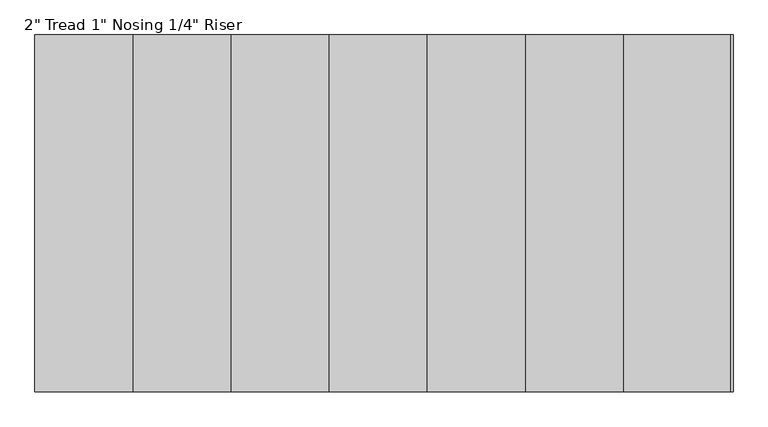
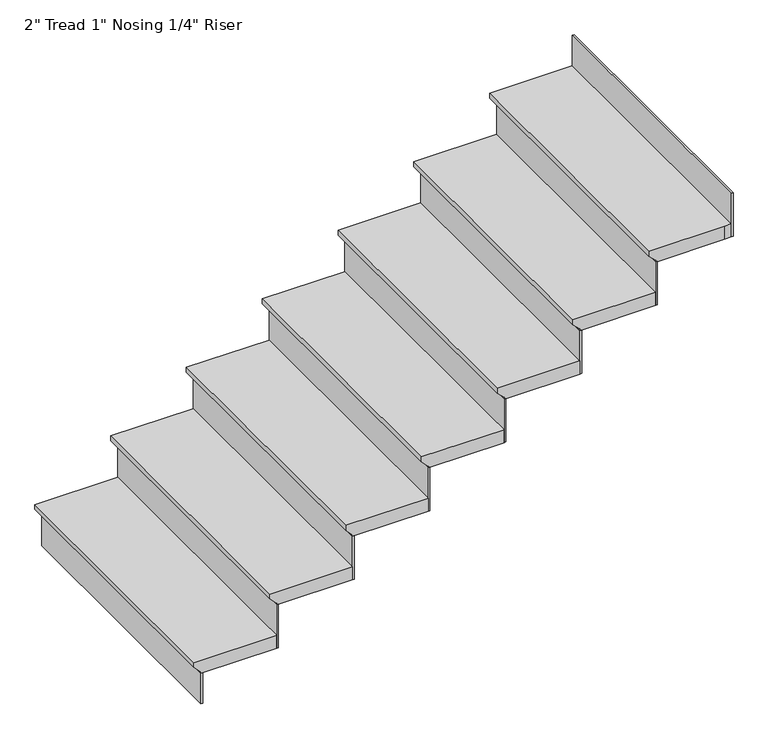
"""IFC4 building model written with IfcOpenShell, lengths in millimetres: stair flight geometry."""

from ifc_helpers import new_model, si_unit, origin, place, context, project, spatial, faceted_brep, source, transform, mapped, element, save


def stair_flight_c1e9d316(model_context):
    return source(origin(), model_context, "Body", "Brep", [
        faceted_brep([(-8426.5655018, -682.6966995, 150.2833333), (-8426.5655018, -682.6966995, 169.3333333), (-8426.5655018, 332.8576368, 169.3333333), (-8426.5655018, 332.8576368, 150.2833333), (-8401.1655018, -682.6966995, 124.8833333), (-8401.1655018, 332.8576368, 124.8833333), (-8121.7655018, -682.6966995, 169.3333333), (-8121.7655018, 332.8576368, 169.3333333), (-8401.1655018, 332.8576368, 118.5333333), (-8121.7655018, 332.8576368, 118.5333333), (-8121.7655018, -682.6966995, 118.5333333), (-8401.1655018, -682.6966995, 118.5333333)], [[[0, 1, 2, 3]], [[4, 0, 3, 5]], [[2, 1, 6, 7]], [[8, 9, 10, 11]], [[2, 7, 9, 8, 5, 3]], [[8, 11, 4, 5]], [[6, 1, 0, 4, 11, 10]], [[7, 6, 10, 9]]]),
        faceted_brep([(-8401.1655018, -682.6966995, 118.5333333), (-8401.1655018, -682.6966995, 0.0), (-8394.8155018, -682.6966995, 0.0), (-8394.8155018, -682.6966995, 118.5333333), (-8401.1655018, 332.8576368, 118.5333333), (-8394.8155018, 332.8576368, 118.5333333), (-8394.8155018, 332.8576368, 0.0), (-8401.1655018, 332.8576368, 0.0)], [[[0, 1, 2, 3]], [[4, 5, 6, 7]], [[1, 0, 4, 7]], [[2, 1, 7, 6]], [[3, 2, 6, 5]], [[0, 3, 5, 4]]]),
        faceted_brep([(-6445.3655018, -682.6966995, 1303.8666667), (-6445.3655018, -682.6966995, 1134.5333333), (-6439.0155018, -682.6966995, 1134.5333333), (-6439.0155018, -682.6966995, 1303.8666667), (-6445.3655018, 332.8576368, 1303.8666667), (-6439.0155018, 332.8576368, 1303.8666667), (-6439.0155018, 332.8576368, 1134.5333333), (-6445.3655018, 332.8576368, 1134.5333333)], [[[0, 1, 2, 3]], [[4, 5, 6, 7]], [[1, 0, 4, 7]], [[2, 1, 7, 6]], [[3, 2, 6, 5]], [[0, 3, 5, 4]]]),
        faceted_brep([(-8121.7655018, -682.6966995, 287.8666667), (-8121.7655018, -682.6966995, 118.5333333), (-8115.4155018, -682.6966995, 118.5333333), (-8115.4155018, -682.6966995, 287.8666667), (-8121.7655018, 332.8576368, 287.8666667), (-8115.4155018, 332.8576368, 287.8666667), (-8115.4155018, 332.8576368, 118.5333333), (-8121.7655018, 332.8576368, 118.5333333)], [[[0, 1, 2, 3]], [[4, 5, 6, 7]], [[1, 0, 4, 7]], [[2, 1, 7, 6]], [[3, 2, 6, 5]], [[0, 3, 5, 4]]]),
        faceted_brep([(-8147.1655018, 332.8576368, 338.6666667), (-8147.1655018, -682.6966995, 338.6666667), (-7842.3655018, -682.6966995, 338.6666667), (-7842.3655018, 332.8576368, 338.6666667), (-8121.7655018, 332.8576368, 287.8666667), (-7842.3655018, 332.8576368, 287.8666667), (-7842.3655018, -682.6966995, 287.8666667), (-8121.7655018, -682.6966995, 287.8666667), (-8121.7655018, 332.8576368, 294.2166667), (-8147.1655018, 332.8576368, 319.6166667), (-8121.7655018, -682.6966995, 294.2166667), (-8147.1655018, -682.6966995, 319.6166667)], [[[0, 1, 2, 3]], [[4, 5, 6, 7]], [[0, 3, 5, 4, 8, 9]], [[4, 7, 10, 8]], [[2, 1, 11, 10, 7, 6]], [[3, 2, 6, 5]], [[11, 1, 0, 9]], [[10, 11, 9, 8]]]),
        faceted_brep([(-7842.3655018, -682.6966995, 457.2), (-7842.3655018, -682.6966995, 287.8666667), (-7836.0155018, -682.6966995, 287.8666667), (-7836.0155018, -682.6966995, 457.2), (-7842.3655018, 332.8576368, 457.2), (-7836.0155018, 332.8576368, 457.2), (-7836.0155018, 332.8576368, 287.8666667), (-7842.3655018, 332.8576368, 287.8666667)], [[[0, 1, 2, 3]], [[4, 5, 6, 7]], [[1, 0, 4, 7]], [[2, 1, 7, 6]], [[3, 2, 6, 5]], [[0, 3, 5, 4]]]),
        faceted_brep([(-7867.7655018, 332.8576368, 508.0), (-7867.7655018, -682.6966995, 508.0), (-7562.9655018, -682.6966995, 508.0), (-7562.9655018, 332.8576368, 508.0), (-7842.3655018, 332.8576368, 457.2), (-7562.9655018, 332.8576368, 457.2), (-7562.9655018, -682.6966995, 457.2), (-7842.3655018, -682.6966995, 457.2), (-7842.3655018, 332.8576368, 463.55), (-7867.7655018, 332.8576368, 488.95), (-7842.3655018, -682.6966995, 463.55), (-7867.7655018, -682.6966995, 488.95)], [[[0, 1, 2, 3]], [[4, 5, 6, 7]], [[0, 3, 5, 4, 8, 9]], [[4, 7, 10, 8]], [[2, 1, 11, 10, 7, 6]], [[3, 2, 6, 5]], [[11, 1, 0, 9]], [[10, 11, 9, 8]]]),
        faceted_brep([(-7562.9655018, -682.6966995, 626.5333333), (-7562.9655018, -682.6966995, 457.2), (-7556.6155018, -682.6966995, 457.2), (-7556.6155018, -682.6966995, 626.5333333), (-7562.9655018, 332.8576368, 626.5333333), (-7556.6155018, 332.8576368, 626.5333333), (-7556.6155018, 332.8576368, 457.2), (-7562.9655018, 332.8576368, 457.2)], [[[0, 1, 2, 3]], [[4, 5, 6, 7]], [[1, 0, 4, 7]], [[2, 1, 7, 6]], [[3, 2, 6, 5]], [[0, 3, 5, 4]]]),
        faceted_brep([(-7588.3655018, 332.8576368, 677.3333333), (-7588.3655018, -682.6966995, 677.3333333), (-7283.5655018, -682.6966995, 677.3333333), (-7283.5655018, 332.8576368, 677.3333333), (-7562.9655018, 332.8576368, 626.5333333), (-7283.5655018, 332.8576368, 626.5333333), (-7283.5655018, -682.6966995, 626.5333333), (-7562.9655018, -682.6966995, 626.5333333), (-7562.9655018, 332.8576368, 632.8833333), (-7588.3655018, 332.8576368, 658.2833333), (-7562.9655018, -682.6966995, 632.8833333), (-7588.3655018, -682.6966995, 658.2833333)], [[[0, 1, 2, 3]], [[4, 5, 6, 7]], [[0, 3, 5, 4, 8, 9]], [[4, 7, 10, 8]], [[2, 1, 11, 10, 7, 6]], [[3, 2, 6, 5]], [[11, 1, 0, 9]], [[10, 11, 9, 8]]]),
        faceted_brep([(-7283.5655018, -682.6966995, 795.8666667), (-7283.5655018, -682.6966995, 626.5333333), (-7277.2155018, -682.6966995, 626.5333333), (-7277.2155018, -682.6966995, 795.8666667), (-7283.5655018, 332.8576368, 795.8666667), (-7277.2155018, 332.8576368, 795.8666667), (-7277.2155018, 332.8576368, 626.5333333), (-7283.5655018, 332.8576368, 626.5333333)], [[[0, 1, 2, 3]], [[4, 5, 6, 7]], [[1, 0, 4, 7]], [[2, 1, 7, 6]], [[3, 2, 6, 5]], [[0, 3, 5, 4]]]),
        faceted_brep([(-7308.9655018, 332.8576368, 846.6666667), (-7308.9655018, -682.6966995, 846.6666667), (-7004.1655018, -682.6966995, 846.6666667), (-7004.1655018, 332.8576368, 846.6666667), (-7283.5655018, 332.8576368, 795.8666667), (-7004.1655018, 332.8576368, 795.8666667), (-7004.1655018, -682.6966995, 795.8666667), (-7283.5655018, -682.6966995, 795.8666667), (-7283.5655018, 332.8576368, 802.2166667), (-7308.9655018, 332.8576368, 827.6166667), (-7283.5655018, -682.6966995, 802.2166667), (-7308.9655018, -682.6966995, 827.6166667)], [[[0, 1, 2, 3]], [[4, 5, 6, 7]], [[0, 3, 5, 4, 8, 9]], [[4, 7, 10, 8]], [[2, 1, 11, 10, 7, 6]], [[3, 2, 6, 5]], [[11, 1, 0, 9]], [[10, 11, 9, 8]]]),
        faceted_brep([(-7004.1655018, -682.6966995, 965.2), (-7004.1655018, -682.6966995, 795.8666667), (-6997.8155018, -682.6966995, 795.8666667), (-6997.8155018, -682.6966995, 965.2), (-7004.1655018, 332.8576368, 965.2), (-6997.8155018, 332.8576368, 965.2), (-6997.8155018, 332.8576368, 795.8666667), (-7004.1655018, 332.8576368, 795.8666667)], [[[0, 1, 2, 3]], [[4, 5, 6, 7]], [[1, 0, 4, 7]], [[2, 1, 7, 6]], [[3, 2, 6, 5]], [[0, 3, 5, 4]]]),
        faceted_brep([(-7029.5655018, 332.8576368, 1016.0), (-7029.5655018, -682.6966995, 1016.0), (-6724.7655018, -682.6966995, 1016.0), (-6724.7655018, 332.8576368, 1016.0), (-7004.1655018, 332.8576368, 965.2), (-6724.7655018, 332.8576368, 965.2), (-6724.7655018, -682.6966995, 965.2), (-7004.1655018, -682.6966995, 965.2), (-7004.1655018, 332.8576368, 971.55), (-7029.5655018, 332.8576368, 996.95), (-7004.1655018, -682.6966995, 971.55), (-7029.5655018, -682.6966995, 996.95)], [[[0, 1, 2, 3]], [[4, 5, 6, 7]], [[0, 3, 5, 4, 8, 9]], [[4, 7, 10, 8]], [[2, 1, 11, 10, 7, 6]], [[3, 2, 6, 5]], [[11, 1, 0, 9]], [[10, 11, 9, 8]]]),
        faceted_brep([(-6724.7655018, -682.6966995, 1134.5333333), (-6724.7655018, -682.6966995, 965.2), (-6718.4155018, -682.6966995, 965.2), (-6718.4155018, -682.6966995, 1134.5333333), (-6724.7655018, 332.8576368, 1134.5333333), (-6718.4155018, 332.8576368, 1134.5333333), (-6718.4155018, 332.8576368, 965.2), (-6724.7655018, 332.8576368, 965.2)], [[[0, 1, 2, 3]], [[4, 5, 6, 7]], [[1, 0, 4, 7]], [[2, 1, 7, 6]], [[3, 2, 6, 5]], [[0, 3, 5, 4]]]),
        faceted_brep([(-6750.1655018, 332.8576368, 1185.3333333), (-6750.1655018, -682.6966995, 1185.3333333), (-6470.7655018, -682.6966995, 1185.3333333), (-6445.3655018, -682.6966995, 1185.3333333), (-6445.3655018, 332.8576368, 1185.3333333), (-6724.7655018, 332.8576368, 1134.5333333), (-6445.3655018, 332.8576368, 1134.5333333), (-6445.3655018, -682.6966995, 1134.5333333), (-6470.7655018, -682.6966995, 1134.5333333), (-6724.7655018, -682.6966995, 1134.5333333), (-6724.7655018, 332.8576368, 1140.8833333), (-6750.1655018, 332.8576368, 1166.2833333), (-6724.7655018, -682.6966995, 1140.8833333), (-6750.1655018, -682.6966995, 1166.2833333)], [[[0, 1, 2, 3, 4]], [[5, 6, 7, 8, 9]], [[0, 4, 6, 5, 10, 11]], [[5, 9, 12, 10]], [[2, 1, 13, 12, 9, 8]], [[3, 2, 8, 7]], [[4, 3, 7, 6]], [[13, 1, 0, 11]], [[12, 13, 11, 10]]]),
    ])


if __name__ == "__main__":
    model = new_model("IFC4")
    model_context = context("Model", 3, world=origin())
    ifc_project = project(units=[si_unit("LENGTHUNIT", "METRE", prefix="MILLI")], contexts=[model_context])
    site = spatial("IfcSite", under=ifc_project)
    building = spatial("IfcBuilding", under=site)
    placement = place(None, origin())
    stair_flight_shape = stair_flight_c1e9d316(model_context)
    element("IfcStairFlight", 1, ObjectType="2\" Tread 1\" Nosing 1/4\" Riser", at=placement, inside=building, context=model_context, shape_type="MappedRepresentation", body=[
        mapped(stair_flight_shape, transform((0.0, 0.0, 0.0), x_axis=(1.0, 0.0, 0.0), y_axis=(0.0, 1.0, 0.0), z_axis=(0.0, 0.0, 1.0))),
    ])
    save(model, "model.ifc")
